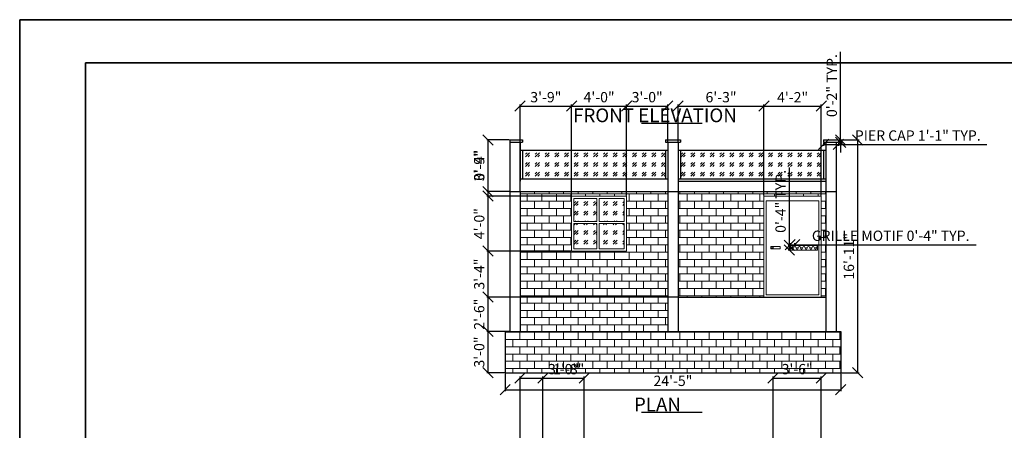
# Model space of a CAD drawing. Units: inches. Extents: x 1798 to 3594, y 1405 to 2404.
# Tile 5 of 6: x 1798 to 2658, y 2046 to 2404. Entities that reach past the tile are written whole.
import ezdxf

# ---------------------------------------------------------------- set-up
doc = ezdxf.new("R2010")
doc.units = ezdxf.units.IN
for name, color, linetype, lineweight in [('A-ANNO-DIMS', 6, 'Continuous', 18), ('A-ANNO-TITL', 6, 'Continuous', 25), ('A-ANNO-TTLB', 7, 'Continuous', 35), ('A-DOOR', 3, 'Continuous', 18), ('A-ELEV', 7, 'Continuous', 30), ('A-GLAZ', 4, 'Continuous', 18), ('A-GLAZ-PATT', 252, 'Continuous', 13), ('A-WALL-PATT', 252, 'Continuous', 13)]:
    doc.layers.add(name, color=color, linetype=linetype, lineweight=lineweight)
doc.styles.get("Standard").update_dxf_attribs({"font": 'arial.ttf'})
doc.dimstyles.new('ISO-25', dxfattribs={"dimtxt": 9, "dimasz": 9, "dimexe": 1.25, "dimexo": 0.625, "dimgap": 2, "dimtad": 1, "dimdec": 1, "dimlunit": 4, "dimtxsty": 'Standard', "dimblk": 'OBLIQUE', "dimcen": 2.5, "dimazin": 0, "dimtfac": 1, "dimtdec": 1, "dimtmove": 0, "dimatfit": 3, "dimfxl": 1, "dimarcsym": 0})
pattern_1 = [(45, (0, 1019.875), (8.485281, 0), [5, -7]), (45, (2.1213, 1019.875), (8.485281, 0), [2, -10]), (45, (0, 1021.996), (8.485281, 0), [2, -10])]

# ---------------------------------------------------------------- blocks, each defined once
blk = doc.blocks.new('PIER-CAP-13-ELEV')
for p, q in [((0, 2), (13, 2)), ((0, 2), (0, 0)), ((0, 0), (13, 0)), ((13, 2), (13, 0))]:
    blk.add_line(p, q)
blk = doc.blocks.new('DOOR-GRILLE-V-MOTIF')
for p, q in [((0, 4), (2, 0)), ((1, 2), (3, 2)), ((2, 0), (4, 4))]:
    blk.add_line(p, q)
blk = doc.blocks.new('_Oblique')
at = {"color": 0, "linetype": 'ByBlock', "lineweight": -2}
blk.add_line((-0.5, -0.5), (0.5, 0.5), dxfattribs=at)
blk = doc.blocks.new('*D15')
at = {"layer": 'A-ANNO-DIMS', "color": 0, "lineweight": -2, "transparency": 16777216}
for p, q in [((2471.14, 2207.46), (2471.14, 2208.69)), ((2471.14, 2207.44), (2475.14, 2207.44)), ((2475.14, 2207.46), (2475.14, 2208.69)), ((2475.14, 2207.44), (2633.67, 2207.44))]:
    blk.add_line(p, q, dxfattribs=at)
at = {"layer": 'Defpoints', "color": 0, "transparency": 16777216}
for p in [(2471.14, 2206.84), (2475.14, 2207.44), (2475.14, 2206.84)]:
    blk.add_point(p, dxfattribs=at)
at = {"layer": 'A-ANNO-DIMS', "color": 0, "lineweight": -2, "transparency": 16777216, "xscale": 9, "yscale": 9, "zscale": 9, "rotation": 180}
blk.add_blockref('_Oblique', (2471.14, 2207.44), dxfattribs=at)
at = {"layer": 'A-ANNO-DIMS', "color": 0, "lineweight": -2, "transparency": 16777216, "xscale": 9, "yscale": 9, "zscale": 9}
blk.add_blockref('_Oblique', (2475.14, 2207.44), dxfattribs=at)
at = {"layer": 'A-ANNO-DIMS', "color": 0, "transparency": 16777216, "insert": (2558.91, 2214.09), "char_height": 9, "attachment_point": 5}
blk.add_mtext('GRILLE MOTIF 0\'-4" TYP.', dxfattribs=at)
blk = doc.blocks.new('*D16')
at = {"layer": 'A-ANNO-DIMS', "color": 0, "lineweight": -2, "transparency": 16777216}
for p, q in [((2470.54, 2206.84), (2470.54, 2274.7)), ((2470.52, 2206.84), (2469.29, 2206.84)), ((2470.52, 2202.84), (2469.29, 2202.84)), ((2470.54, 2202.84), (2470.54, 2206.84))]:
    blk.add_line(p, q, dxfattribs=at)
at = {"layer": 'Defpoints', "color": 0, "transparency": 16777216}
for p in [(2470.54, 2206.84), (2471.14, 2206.84), (2471.14, 2202.84)]:
    blk.add_point(p, dxfattribs=at)
at = {"layer": 'A-ANNO-DIMS', "color": 0, "lineweight": -2, "transparency": 16777216, "xscale": 9, "yscale": 9, "zscale": 9}
for p, rotation in [((2470.54, 2206.84), 90), ((2470.54, 2202.84), 270)]:
    blk.add_blockref('_Oblique', p, dxfattribs=dict(at, rotation=rotation))
at = {"layer": 'A-ANNO-DIMS', "color": 0, "transparency": 16777216, "insert": (2463.95, 2245.27), "char_height": 9, "attachment_point": 5, "rotation": 90}
blk.add_mtext('0\'-4" TYP.', dxfattribs=at)
blk = doc.blocks.new('*D21')
at = {"layer": 'A-ANNO-DIMS', "color": 0, "lineweight": -2, "transparency": 16777216}
for p, q in [((2500.27, 2296.21), (2500.27, 2293.64)), ((2513.27, 2296.21), (2513.27, 2293.64)), ((2500.27, 2294.89), (2513.27, 2294.89)), ((2513.27, 2294.89), (2642.87, 2294.89))]:
    blk.add_line(p, q, dxfattribs=at)
at = {"layer": 'Defpoints', "color": 0, "transparency": 16777216}
for p in [(2500.27, 2296.84), (2513.27, 2296.84), (2513.27, 2294.89)]:
    blk.add_point(p, dxfattribs=at)
at = {"layer": 'A-ANNO-DIMS', "color": 0, "lineweight": -2, "transparency": 16777216, "xscale": 9, "yscale": 9, "zscale": 9, "rotation": 180}
blk.add_blockref('_Oblique', (2500.27, 2294.89), dxfattribs=at)
at = {"layer": 'A-ANNO-DIMS', "color": 0, "lineweight": -2, "transparency": 16777216, "xscale": 9, "yscale": 9, "zscale": 9}
blk.add_blockref('_Oblique', (2513.27, 2294.89), dxfattribs=at)
at = {"layer": 'A-ANNO-DIMS', "color": 0, "transparency": 16777216, "insert": (2582.57, 2301.54), "char_height": 9, "attachment_point": 5}
blk.add_mtext('PIER CAP 1\'-1" TYP.', dxfattribs=at)
blk = doc.blocks.new('*D22')
at = {"layer": 'A-ANNO-DIMS', "color": 0, "lineweight": -2, "transparency": 16777216}
for p, q in [((2515.22, 2298.84), (2515.22, 2375.7)), ((2513.9, 2298.84), (2516.47, 2298.84)), ((2513.9, 2296.84), (2516.47, 2296.84)), ((2515.22, 2296.84), (2515.22, 2298.84)), ((2515.22, 2296.84), (2515.22, 2287.84))]:
    blk.add_line(p, q, dxfattribs=at)
at = {"layer": 'Defpoints', "color": 0, "transparency": 16777216}
for p in [(2513.27, 2298.84), (2513.27, 2296.84), (2515.22, 2298.84)]:
    blk.add_point(p, dxfattribs=at)
at = {"layer": 'A-ANNO-DIMS', "color": 0, "lineweight": -2, "transparency": 16777216, "xscale": 9, "yscale": 9, "zscale": 9}
for p, rotation in [((2515.22, 2298.84), 270), ((2515.22, 2296.84), 90)]:
    blk.add_blockref('_Oblique', p, dxfattribs=dict(at, rotation=rotation))
at = {"layer": 'A-ANNO-DIMS', "color": 0, "transparency": 16777216, "insert": (2508.63, 2346.27), "char_height": 9, "attachment_point": 5, "rotation": 90}
blk.add_mtext('0\'-2" TYP.', dxfattribs=at)
blk = doc.blocks.new('*D42')
at = {"layer": 'A-ANNO-DIMS', "color": 0, "lineweight": -2, "transparency": 16777216}
for p, q in [((2235.27, 1867.44), (2235.27, 2092.43)), ((2235.27, 2091.18), (2255.27, 2091.18)), ((2255.27, 1867.44), (2255.27, 2092.43)), ((2255.27, 2091.18), (2291.35, 2091.18))]:
    blk.add_line(p, q, dxfattribs=at)
at = {"layer": 'Defpoints', "color": 0, "transparency": 16777216}
for p in [(2255.27, 2091.18), (2235.27, 1866.81), (2255.27, 1866.81)]:
    blk.add_point(p, dxfattribs=at)
at = {"layer": 'A-ANNO-DIMS', "color": 0, "lineweight": -2, "transparency": 16777216, "xscale": 9, "yscale": 9, "zscale": 9, "rotation": 180}
blk.add_blockref('_Oblique', (2235.27, 2091.18), dxfattribs=at)
at = {"layer": 'A-ANNO-DIMS', "color": 0, "lineweight": -2, "transparency": 16777216, "xscale": 9, "yscale": 9, "zscale": 9}
blk.add_blockref('_Oblique', (2255.27, 2091.18), dxfattribs=at)
at = {"layer": 'A-ANNO-DIMS', "color": 0, "transparency": 16777216, "insert": (2277.81, 2097.78), "char_height": 9, "attachment_point": 5}
blk.add_mtext('1\'-8"', dxfattribs=at)
blk = doc.blocks.new('*D43')
at = {"layer": 'A-ANNO-DIMS', "color": 0, "lineweight": -2, "transparency": 16777216}
for p, q in [((2255.27, 1867.44), (2255.27, 2092.43)), ((2255.27, 2091.18), (2291.27, 2091.18)), ((2291.27, 1867.44), (2291.27, 2092.43))]:
    blk.add_line(p, q, dxfattribs=at)
at = {"layer": 'Defpoints', "color": 0, "transparency": 16777216}
for p in [(2291.27, 2091.18), (2255.27, 1866.81), (2291.27, 1866.81)]:
    blk.add_point(p, dxfattribs=at)
at = {"layer": 'A-ANNO-DIMS', "color": 0, "lineweight": -2, "transparency": 16777216, "xscale": 9, "yscale": 9, "zscale": 9, "rotation": 180}
blk.add_blockref('_Oblique', (2255.27, 2091.18), dxfattribs=at)
at = {"layer": 'A-ANNO-DIMS', "color": 0, "lineweight": -2, "transparency": 16777216, "xscale": 9, "yscale": 9, "zscale": 9}
blk.add_blockref('_Oblique', (2291.27, 2091.18), dxfattribs=at)
at = {"layer": 'A-ANNO-DIMS', "color": 0, "transparency": 16777216, "insert": (2273.27, 2097.78), "char_height": 9, "attachment_point": 5}
blk.add_mtext('3\'-0"', dxfattribs=at)
blk = doc.blocks.new('*D47')
at = {"layer": 'A-ANNO-DIMS', "color": 0, "lineweight": -2, "transparency": 16777216}
for p, q in [((2456.27, 1666.44), (2456.27, 2092.43)), ((2456.27, 2091.18), (2498.27, 2091.18)), ((2498.27, 1666.44), (2498.27, 2092.43))]:
    blk.add_line(p, q, dxfattribs=at)
at = {"layer": 'Defpoints', "color": 0, "transparency": 16777216}
for p in [(2498.27, 2091.18), (2456.27, 1665.81), (2498.27, 1665.81)]:
    blk.add_point(p, dxfattribs=at)
at = {"layer": 'A-ANNO-DIMS', "color": 0, "lineweight": -2, "transparency": 16777216, "xscale": 9, "yscale": 9, "zscale": 9, "rotation": 180}
blk.add_blockref('_Oblique', (2456.27, 2091.18), dxfattribs=at)
at = {"layer": 'A-ANNO-DIMS', "color": 0, "lineweight": -2, "transparency": 16777216, "xscale": 9, "yscale": 9, "zscale": 9}
blk.add_blockref('_Oblique', (2498.27, 2091.18), dxfattribs=at)
at = {"layer": 'A-ANNO-DIMS', "color": 0, "transparency": 16777216, "insert": (2477.27, 2097.78), "char_height": 9, "attachment_point": 5}
blk.add_mtext('3\'-6"', dxfattribs=at)
blk = doc.blocks.new('*D53')
at = {"layer": 'A-ANNO-DIMS', "color": 0, "lineweight": -2, "transparency": 16777216}
for p, q in [((2222.27, 2095.21), (2222.27, 2079.69)), ((2515.27, 2095.21), (2515.27, 2079.69)), ((2222.27, 2080.94), (2515.27, 2080.94))]:
    blk.add_line(p, q, dxfattribs=at)
at = {"layer": 'Defpoints', "color": 0, "transparency": 16777216}
for p in [(2222.27, 2095.84), (2515.27, 2095.84), (2515.27, 2080.94)]:
    blk.add_point(p, dxfattribs=at)
at = {"layer": 'A-ANNO-DIMS', "color": 0, "lineweight": -2, "transparency": 16777216, "xscale": 9, "yscale": 9, "zscale": 9, "rotation": 180}
blk.add_blockref('_Oblique', (2222.27, 2080.94), dxfattribs=at)
at = {"layer": 'A-ANNO-DIMS', "color": 0, "lineweight": -2, "transparency": 16777216, "xscale": 9, "yscale": 9, "zscale": 9}
blk.add_blockref('_Oblique', (2515.27, 2080.94), dxfattribs=at)
at = {"layer": 'A-ANNO-DIMS', "color": 0, "transparency": 16777216, "insert": (2368.77, 2087.53), "char_height": 9, "attachment_point": 5}
blk.add_mtext('24\'-5"', dxfattribs=at)
blk = doc.blocks.new('*D54')
at = {"layer": 'A-ANNO-DIMS', "color": 0, "lineweight": -2, "transparency": 16777216}
for p, q in [((2513.9, 2298.84), (2531.42, 2298.84)), ((2530.17, 2095.84), (2530.17, 2298.84)), ((2515.9, 2095.84), (2531.42, 2095.84))]:
    blk.add_line(p, q, dxfattribs=at)
at = {"layer": 'Defpoints', "color": 0, "transparency": 16777216}
for p in [(2513.27, 2298.84), (2530.17, 2298.84), (2515.27, 2095.84)]:
    blk.add_point(p, dxfattribs=at)
at = {"layer": 'A-ANNO-DIMS', "color": 0, "lineweight": -2, "transparency": 16777216, "xscale": 9, "yscale": 9, "zscale": 9}
for p, rotation in [((2530.17, 2298.84), 90), ((2530.17, 2095.84), 270)]:
    blk.add_blockref('_Oblique', p, dxfattribs=dict(at, rotation=rotation))
at = {"layer": 'A-ANNO-DIMS', "color": 0, "transparency": 16777216, "insert": (2523.58, 2197.34), "char_height": 9, "attachment_point": 5, "rotation": 90}
blk.add_mtext('16\'-11"', dxfattribs=at)
blk = doc.blocks.new('*D55')
at = {"layer": 'A-ANNO-DIMS', "color": 0, "lineweight": -2, "transparency": 16777216}
for p, q in [((2221.65, 2131.84), (2206.12, 2131.84)), ((2207.37, 2095.84), (2207.37, 2131.84)), ((2221.65, 2095.84), (2206.12, 2095.84))]:
    blk.add_line(p, q, dxfattribs=at)
at = {"layer": 'Defpoints', "color": 0, "transparency": 16777216}
for p in [(2207.37, 2131.84), (2222.27, 2131.84), (2222.27, 2095.84)]:
    blk.add_point(p, dxfattribs=at)
at = {"layer": 'A-ANNO-DIMS', "color": 0, "lineweight": -2, "transparency": 16777216, "xscale": 9, "yscale": 9, "zscale": 9}
for p, rotation in [((2207.37, 2131.84), 90), ((2207.37, 2095.84), 270)]:
    blk.add_blockref('_Oblique', p, dxfattribs=dict(at, rotation=rotation))
at = {"layer": 'A-ANNO-DIMS', "color": 0, "transparency": 16777216, "insert": (2200.77, 2113.84), "char_height": 9, "attachment_point": 5, "rotation": 90}
blk.add_mtext('3\'-0"', dxfattribs=at)
blk = doc.blocks.new('*D56')
at = {"layer": 'A-ANNO-DIMS', "color": 0, "lineweight": -2, "transparency": 16777216}
for p, q in [((2372.65, 2161.84), (2206.12, 2161.84)), ((2207.37, 2131.84), (2207.37, 2161.84)), ((2225.65, 2131.84), (2206.12, 2131.84))]:
    blk.add_line(p, q, dxfattribs=at)
at = {"layer": 'Defpoints', "color": 0, "transparency": 16777216}
for p in [(2207.37, 2161.84), (2373.27, 2161.84), (2226.27, 2131.84)]:
    blk.add_point(p, dxfattribs=at)
at = {"layer": 'A-ANNO-DIMS', "color": 0, "lineweight": -2, "transparency": 16777216, "xscale": 9, "yscale": 9, "zscale": 9}
for p, rotation in [((2207.37, 2161.84), 90), ((2207.37, 2131.84), 270)]:
    blk.add_blockref('_Oblique', p, dxfattribs=dict(at, rotation=rotation))
at = {"layer": 'A-ANNO-DIMS', "color": 0, "transparency": 16777216, "insert": (2200.78, 2146.84), "char_height": 9, "attachment_point": 5, "rotation": 90}
blk.add_mtext('2\'-6"', dxfattribs=at)
blk = doc.blocks.new('*D57')
at = {"layer": 'A-ANNO-DIMS', "color": 0, "lineweight": -2, "transparency": 16777216}
for p, q in [((2279.65, 2201.84), (2206.12, 2201.84)), ((2207.37, 2161.84), (2207.37, 2201.84)), ((2372.65, 2161.84), (2206.12, 2161.84))]:
    blk.add_line(p, q, dxfattribs=at)
at = {"layer": 'Defpoints', "color": 0, "transparency": 16777216}
for p in [(2207.37, 2201.84), (2280.27, 2201.84), (2373.27, 2161.84)]:
    blk.add_point(p, dxfattribs=at)
at = {"layer": 'A-ANNO-DIMS', "color": 0, "lineweight": -2, "transparency": 16777216, "xscale": 9, "yscale": 9, "zscale": 9}
for p, rotation in [((2207.37, 2201.84), 90), ((2207.37, 2161.84), 270)]:
    blk.add_blockref('_Oblique', p, dxfattribs=dict(at, rotation=rotation))
at = {"layer": 'A-ANNO-DIMS', "color": 0, "transparency": 16777216, "insert": (2200.77, 2181.84), "char_height": 9, "attachment_point": 5, "rotation": 90}
blk.add_mtext('3\'-4"', dxfattribs=at)
blk = doc.blocks.new('*D58')
at = {"layer": 'A-ANNO-DIMS', "color": 0, "lineweight": -2, "transparency": 16777216}
for p, q in [((2279.65, 2249.84), (2206.12, 2249.84)), ((2207.37, 2201.84), (2207.37, 2249.84)), ((2279.65, 2201.84), (2206.12, 2201.84))]:
    blk.add_line(p, q, dxfattribs=at)
at = {"layer": 'Defpoints', "color": 0, "transparency": 16777216}
for p in [(2207.37, 2249.84), (2280.27, 2249.84), (2280.27, 2201.84)]:
    blk.add_point(p, dxfattribs=at)
at = {"layer": 'A-ANNO-DIMS', "color": 0, "lineweight": -2, "transparency": 16777216, "xscale": 9, "yscale": 9, "zscale": 9}
for p, rotation in [((2207.37, 2249.84), 90), ((2207.37, 2201.84), 270)]:
    blk.add_blockref('_Oblique', p, dxfattribs=dict(at, rotation=rotation))
at = {"layer": 'A-ANNO-DIMS', "color": 0, "transparency": 16777216, "insert": (2200.78, 2225.84), "char_height": 9, "attachment_point": 5, "rotation": 90}
blk.add_mtext('4\'-0"', dxfattribs=at)
blk = doc.blocks.new('*D59')
at = {"layer": 'A-ANNO-DIMS', "color": 0, "lineweight": -2, "transparency": 16777216}
for p, q in [((2207.37, 2253.84), (2207.37, 2290.76)), ((2225.65, 2253.84), (2206.12, 2253.84)), ((2207.37, 2249.84), (2207.37, 2253.84)), ((2279.65, 2249.84), (2206.12, 2249.84))]:
    blk.add_line(p, q, dxfattribs=at)
at = {"layer": 'Defpoints', "color": 0, "transparency": 16777216}
for p in [(2207.37, 2253.84), (2226.27, 2253.84), (2280.27, 2249.84)]:
    blk.add_point(p, dxfattribs=at)
at = {"layer": 'A-ANNO-DIMS', "color": 0, "lineweight": -2, "transparency": 16777216, "xscale": 9, "yscale": 9, "zscale": 9}
for p, rotation in [((2207.37, 2253.84), 90), ((2207.37, 2249.84), 270)]:
    blk.add_blockref('_Oblique', p, dxfattribs=dict(at, rotation=rotation))
at = {"layer": 'A-ANNO-DIMS', "color": 0, "transparency": 16777216, "insert": (2200.78, 2276.8), "char_height": 9, "attachment_point": 5, "rotation": 90}
blk.add_mtext('0\'-4"', dxfattribs=at)
blk = doc.blocks.new('*D60')
at = {"layer": 'A-ANNO-DIMS', "color": 0, "lineweight": -2, "transparency": 16777216}
for p, q in [((2225.65, 2298.84), (2206.12, 2298.84)), ((2207.37, 2253.84), (2207.37, 2298.84)), ((2225.65, 2253.84), (2206.12, 2253.84))]:
    blk.add_line(p, q, dxfattribs=at)
at = {"layer": 'Defpoints', "color": 0, "transparency": 16777216}
for p in [(2207.37, 2298.84), (2226.27, 2298.84), (2226.27, 2253.84)]:
    blk.add_point(p, dxfattribs=at)
at = {"layer": 'A-ANNO-DIMS', "color": 0, "lineweight": -2, "transparency": 16777216, "xscale": 9, "yscale": 9, "zscale": 9}
for p, rotation in [((2207.37, 2298.84), 90), ((2207.37, 2253.84), 270)]:
    blk.add_blockref('_Oblique', p, dxfattribs=dict(at, rotation=rotation))
at = {"layer": 'A-ANNO-DIMS', "color": 0, "transparency": 16777216, "insert": (2200.77, 2276.34), "char_height": 9, "attachment_point": 5, "rotation": 90}
blk.add_mtext('3\'-9"', dxfattribs=at)
blk = doc.blocks.new('*D61')
at = {"layer": 'A-ANNO-DIMS', "color": 0, "lineweight": -2, "transparency": 16777216}
for p, q in [((2235.27, 2254.46), (2235.27, 2329.66)), ((2235.27, 2328.41), (2280.27, 2328.41)), ((2280.27, 2250.46), (2280.27, 2329.66))]:
    blk.add_line(p, q, dxfattribs=at)
at = {"layer": 'Defpoints', "color": 0, "transparency": 16777216}
for p in [(2280.27, 2328.41), (2235.27, 2253.84), (2280.27, 2249.84)]:
    blk.add_point(p, dxfattribs=at)
at = {"layer": 'A-ANNO-DIMS', "color": 0, "lineweight": -2, "transparency": 16777216, "xscale": 9, "yscale": 9, "zscale": 9, "rotation": 180}
blk.add_blockref('_Oblique', (2235.27, 2328.41), dxfattribs=at)
at = {"layer": 'A-ANNO-DIMS', "color": 0, "lineweight": -2, "transparency": 16777216, "xscale": 9, "yscale": 9, "zscale": 9}
blk.add_blockref('_Oblique', (2280.27, 2328.41), dxfattribs=at)
at = {"layer": 'A-ANNO-DIMS', "color": 0, "transparency": 16777216, "insert": (2257.77, 2335.01), "char_height": 9, "attachment_point": 5}
blk.add_mtext('3\'-9"', dxfattribs=at)
blk = doc.blocks.new('*D62')
at = {"layer": 'A-ANNO-DIMS', "color": 0, "lineweight": -2, "transparency": 16777216}
for p, q in [((2280.27, 2250.46), (2280.27, 2329.66)), ((2280.27, 2328.41), (2328.27, 2328.41)), ((2328.27, 2250.46), (2328.27, 2329.66))]:
    blk.add_line(p, q, dxfattribs=at)
at = {"layer": 'Defpoints', "color": 0, "transparency": 16777216}
for p in [(2328.27, 2328.41), (2280.27, 2249.84), (2328.27, 2249.84)]:
    blk.add_point(p, dxfattribs=at)
at = {"layer": 'A-ANNO-DIMS', "color": 0, "lineweight": -2, "transparency": 16777216, "xscale": 9, "yscale": 9, "zscale": 9, "rotation": 180}
blk.add_blockref('_Oblique', (2280.27, 2328.41), dxfattribs=at)
at = {"layer": 'A-ANNO-DIMS', "color": 0, "lineweight": -2, "transparency": 16777216, "xscale": 9, "yscale": 9, "zscale": 9}
blk.add_blockref('_Oblique', (2328.27, 2328.41), dxfattribs=at)
at = {"layer": 'A-ANNO-DIMS', "color": 0, "transparency": 16777216, "insert": (2304.27, 2335.01), "char_height": 9, "attachment_point": 5}
blk.add_mtext('4\'-0"', dxfattribs=at)
blk = doc.blocks.new('*D63')
at = {"layer": 'A-ANNO-DIMS', "color": 0, "lineweight": -2, "transparency": 16777216}
for p, q in [((2328.27, 2250.46), (2328.27, 2329.66)), ((2328.27, 2328.41), (2364.27, 2328.41)), ((2364.27, 2297.46), (2364.27, 2329.66))]:
    blk.add_line(p, q, dxfattribs=at)
at = {"layer": 'Defpoints', "color": 0, "transparency": 16777216}
for p in [(2364.27, 2328.41), (2364.27, 2296.84), (2328.27, 2249.84)]:
    blk.add_point(p, dxfattribs=at)
at = {"layer": 'A-ANNO-DIMS', "color": 0, "lineweight": -2, "transparency": 16777216, "xscale": 9, "yscale": 9, "zscale": 9, "rotation": 180}
blk.add_blockref('_Oblique', (2328.27, 2328.41), dxfattribs=at)
at = {"layer": 'A-ANNO-DIMS', "color": 0, "lineweight": -2, "transparency": 16777216, "xscale": 9, "yscale": 9, "zscale": 9}
blk.add_blockref('_Oblique', (2364.27, 2328.41), dxfattribs=at)
at = {"layer": 'A-ANNO-DIMS', "color": 0, "transparency": 16777216, "insert": (2346.27, 2335.01), "char_height": 9, "attachment_point": 5}
blk.add_mtext('3\'-0"', dxfattribs=at)
blk = doc.blocks.new('*D64')
at = {"layer": 'A-ANNO-DIMS', "color": 0, "lineweight": -2, "transparency": 16777216}
for p, q in [((2373.27, 2297.46), (2373.27, 2329.66)), ((2373.27, 2328.41), (2448.27, 2328.41)), ((2448.27, 2250.46), (2448.27, 2329.66))]:
    blk.add_line(p, q, dxfattribs=at)
at = {"layer": 'Defpoints', "color": 0, "transparency": 16777216}
for p in [(2448.27, 2328.41), (2373.27, 2296.84), (2448.27, 2249.84)]:
    blk.add_point(p, dxfattribs=at)
at = {"layer": 'A-ANNO-DIMS', "color": 0, "lineweight": -2, "transparency": 16777216, "xscale": 9, "yscale": 9, "zscale": 9, "rotation": 180}
blk.add_blockref('_Oblique', (2373.27, 2328.41), dxfattribs=at)
at = {"layer": 'A-ANNO-DIMS', "color": 0, "lineweight": -2, "transparency": 16777216, "xscale": 9, "yscale": 9, "zscale": 9}
blk.add_blockref('_Oblique', (2448.27, 2328.41), dxfattribs=at)
at = {"layer": 'A-ANNO-DIMS', "color": 0, "transparency": 16777216, "insert": (2410.77, 2335.01), "char_height": 9, "attachment_point": 5}
blk.add_mtext('6\'-3"', dxfattribs=at)
blk = doc.blocks.new('*D65')
at = {"layer": 'A-ANNO-DIMS', "color": 0, "lineweight": -2, "transparency": 16777216}
for p, q in [((2448.27, 2250.46), (2448.27, 2329.66)), ((2448.27, 2328.41), (2498.27, 2328.41)), ((2498.27, 2250.46), (2498.27, 2329.66))]:
    blk.add_line(p, q, dxfattribs=at)
at = {"layer": 'Defpoints', "color": 0, "transparency": 16777216}
for p in [(2498.27, 2328.41), (2448.27, 2249.84), (2498.27, 2249.84)]:
    blk.add_point(p, dxfattribs=at)
at = {"layer": 'A-ANNO-DIMS', "color": 0, "lineweight": -2, "transparency": 16777216, "xscale": 9, "yscale": 9, "zscale": 9, "rotation": 180}
blk.add_blockref('_Oblique', (2448.27, 2328.41), dxfattribs=at)
at = {"layer": 'A-ANNO-DIMS', "color": 0, "lineweight": -2, "transparency": 16777216, "xscale": 9, "yscale": 9, "zscale": 9}
blk.add_blockref('_Oblique', (2498.27, 2328.41), dxfattribs=at)
at = {"layer": 'A-ANNO-DIMS', "color": 0, "transparency": 16777216, "insert": (2473.27, 2334.93), "char_height": 9, "attachment_point": 5}
blk.add_mtext('4\'-2"', dxfattribs=at)

msp = doc.modelspace()

# ---------------------------------------------------------------- hatches: boundary and pattern name
at = {"layer": 'A-GLAZ-PATT'}
h = msp.add_hatch(dxfattribs=at)
h.set_pattern_fill('GOST_GLASS', color=256)
h.set_pattern_definition(pattern_1)
h.paths.add_polyline_path([(2237.27, 2289.84), (2237.27, 2264.84), (2362.27, 2264.84), (2362.27, 2289.84)])
h.paths.add_polyline_path([(2375.27, 2289.84), (2375.27, 2264.84), (2500.27, 2264.84), (2500.27, 2289.84)])
h = msp.add_hatch(dxfattribs=at)
h.set_pattern_fill('GOST_GLASS', color=256)
h.set_pattern_definition(pattern_1)
h.paths.add_polyline_path([(2282.27, 2247.84), (2282.27, 2227.84), (2302.27, 2227.84), (2302.27, 2247.84)])
h.paths.add_polyline_path([(2304.27, 2227.84), (2326.27, 2227.84), (2326.27, 2247.84), (2304.27, 2247.84)])
h.paths.add_polyline_path([(2304.27, 2225.84), (2304.27, 2203.84), (2326.27, 2203.84), (2326.27, 2225.84)])
h.paths.add_polyline_path([(2282.27, 2203.84), (2302.27, 2203.84), (2302.27, 2225.84), (2282.27, 2225.84)])
at = {"layer": 'A-WALL-PATT'}
h = msp.add_hatch(dxfattribs=at)
h.set_pattern_fill('BRICK', color=256)
h.set_pattern_definition([(0, (0, 1019.875), (0, 6.35), []), (90, (0, 1019.875), (-12.7, 8e-16), [6.35, -6.35]), (90, (6.35, 1019.875), (-12.7, 8e-16), [-6.35, 6.35])])
h.paths.add_polyline_path([(2515.27, 2131.84), (2222.27, 2131.84), (2222.27, 2095.84), (2515.27, 2095.84)])
h.paths.add_polyline_path([(2364.27, 2253.84), (2235.27, 2253.84), (2235.27, 2131.84), (2364.27, 2131.84)])
h.paths.add_polyline_path([(2280.27, 2201.84), (2280.27, 2249.84), (2328.27, 2249.84), (2328.27, 2201.84)], flags=16)
h.paths.add_polyline_path([(2282.27, 2203.84), (2282.27, 2225.84), (2302.27, 2225.84), (2302.27, 2203.84)], flags=0)
h.paths.add_polyline_path([(2304.27, 2203.84), (2304.27, 2225.84), (2326.27, 2225.84), (2326.27, 2203.84)], flags=0)
h.paths.add_polyline_path([(2282.27, 2227.84), (2282.27, 2247.84), (2302.27, 2247.84), (2302.27, 2227.84)], flags=0)
h.paths.add_polyline_path([(2304.27, 2227.84), (2304.27, 2247.84), (2326.27, 2247.84), (2326.27, 2227.84)], flags=0)
h.paths.add_polyline_path([(2448.27, 2249.84), (2496.27, 2249.84), (2498.27, 2249.84), (2498.27, 2161.84), (2502.27, 2161.84), (2502.27, 2253.84), (2373.27, 2253.84), (2373.27, 2161.84), (2448.27, 2161.84)])

# ---------------------------------------------------------------- linework, layer by layer
at = {"layer": 'A-ANNO-TITL'}
for p, q in [((2341.44, 2313.51), (2394.35, 2313.51)), ((2341.44, 2061.28), (2394.35, 2061.28))]:
    msp.add_line(p, q, dxfattribs=at)
at = {"layer": 'A-ANNO-TTLB'}
for points in [[(1798.35, 2403.73), (3594.23, 2403.73), (3594.23, 1405.28), (1798.35, 1405.28)], [(1855.68, 2366.05), (3540.6, 2366.05), (3540.6, 1444.98), (1855.68, 1444.98)]]:
    msp.add_lwpolyline(points, close=True, dxfattribs=at)
at = {"layer": 'A-DOOR'}
for p, q in [((2448.27, 2249.84), (2448.27, 2161.84)), ((2448.27, 2249.84), (2498.27, 2249.84)), ((2448.27, 2249.84), (2496.27, 2249.84)), ((2450.27, 2245.84), (2450.27, 2163.84)), ((2450.27, 2245.84), (2496.27, 2245.84)), ((2496.27, 2245.84), (2496.27, 2163.84)), ((2498.27, 2249.84), (2498.27, 2161.84)), ((2454.27, 2205.84), (2454.27, 2203.84)), ((2454.27, 2205.84), (2462.27, 2205.84)), ((2454.27, 2204.84), (2456.27, 2204.84)), ((2454.27, 2203.84), (2462.27, 2203.84)), ((2456.27, 2205.84), (2456.27, 2203.84)), ((2456.27, 2205.84), (2456.27, 2203.84)), ((2462.27, 2205.84), (2462.27, 2203.84)), ((2471.14, 2206.84), (2471.14, 2202.84)), ((2471.14, 2206.84), (2495.14, 2206.84)), ((2471.14, 2202.84), (2495.14, 2202.84)), ((2495.14, 2206.84), (2495.14, 2202.84)), ((2450.27, 2163.84), (2496.27, 2163.84))]:
    msp.add_line(p, q, dxfattribs=at)
at = {"layer": 'A-ELEV'}
for p, q in [((2226.27, 2298.84), (2237.27, 2298.84)), ((2226.27, 2298.84), (2226.27, 2131.84)), ((2226.27, 2296.84), (2237.27, 2296.84)), ((2235.27, 2296.84), (2235.27, 2262.84)), ((2237.27, 2298.84), (2237.27, 2296.84)), ((2364.27, 2296.84), (2364.27, 2262.84)), ((2373.27, 2296.84), (2373.27, 2262.84)), ((2502.27, 2296.84), (2502.27, 2262.84)), ((2511.27, 2296.84), (2511.27, 2131.84)), ((2235.27, 2289.84), (2364.27, 2289.84)), ((2237.27, 2289.84), (2237.27, 2264.84)), ((2362.27, 2289.84), (2362.27, 2264.84)), ((2373.27, 2289.84), (2502.27, 2289.84)), ((2375.27, 2289.84), (2375.27, 2264.84)), ((2500.27, 2289.84), (2500.27, 2264.84)), ((2235.27, 2264.84), (2364.27, 2264.84)), ((2364.27, 2262.84), (2364.27, 2131.84)), ((2373.27, 2264.84), (2502.27, 2264.84)), ((2373.27, 2262.84), (2373.27, 2131.84)), ((2373.27, 2262.84), (2502.27, 2262.84)), ((2502.27, 2262.84), (2502.27, 2131.84)), ((2226.27, 2253.84), (2502.27, 2253.84)), ((2235.27, 2253.84), (2235.27, 2131.84)), ((2502.27, 2253.84), (2511.27, 2253.84)), ((2373.27, 2161.84), (2502.27, 2161.84)), ((2222.27, 2131.84), (2515.27, 2131.84)), ((2222.27, 2131.84), (2222.27, 2095.84)), ((2515.27, 2131.84), (2515.27, 2095.84)), ((2222.27, 2095.84), (2515.27, 2095.84))]:
    msp.add_line(p, q, dxfattribs=at)
at = {"layer": 'A-GLAZ'}
for p, q in [((2280.27, 2249.84), (2280.27, 2201.84)), ((2280.27, 2249.84), (2328.27, 2249.84)), ((2282.27, 2247.84), (2302.27, 2247.84)), ((2282.27, 2247.84), (2282.27, 2227.84)), ((2302.27, 2247.84), (2302.27, 2227.84)), ((2304.27, 2247.84), (2304.27, 2227.84)), ((2304.27, 2247.84), (2326.27, 2247.84)), ((2326.27, 2247.84), (2326.27, 2227.84)), ((2328.27, 2249.84), (2328.27, 2201.84)), ((2282.27, 2227.84), (2302.27, 2227.84)), ((2304.27, 2227.84), (2326.27, 2227.84)), ((2282.27, 2225.84), (2302.27, 2225.84)), ((2282.27, 2225.84), (2282.27, 2203.84)), ((2302.27, 2225.84), (2302.27, 2203.84)), ((2304.27, 2225.84), (2326.27, 2225.84)), ((2304.27, 2225.84), (2304.27, 2203.84)), ((2326.27, 2225.84), (2326.27, 2203.84)), ((2280.27, 2201.84), (2328.27, 2201.84)), ((2282.27, 2203.84), (2302.27, 2203.84)), ((2304.27, 2203.84), (2326.27, 2203.84))]:
    msp.add_line(p, q, dxfattribs=at)

# ---------------------------------------------------------------- block references
at = {"layer": 'A-DOOR'}
for p in [(2471.14, 2202.84), (2475.14, 2202.84), (2479.14, 2202.84), (2483.14, 2202.84), (2487.14, 2202.84), (2491.14, 2202.84)]:
    msp.add_blockref('DOOR-GRILLE-V-MOTIF', p, dxfattribs=at)
at = {"layer": 'A-ELEV'}
for p in [(2362.27, 2296.84), (2500.27, 2296.84)]:
    msp.add_blockref('PIER-CAP-13-ELEV', p, dxfattribs=at)

# ---------------------------------------------------------------- texts
at = {"layer": 'A-ANNO-TITL'}
for s, p in [('            FRONT ELEVATION', (2237.55, 2314.34)), ('            PLAN', (2290.72, 2062.11))]:
    msp.add_text(s, height=12, dxfattribs=at).set_placement(p)

# ---------------------------------------------------------------- dimensions: what is measured, and where the dimension line sits
at = {"layer": 'A-ANNO-DIMS'}
for base, p1, p2, picture, middle in [((2515.22, 2298.84), (2513.27, 2296.84), (2513.27, 2298.84), '*D22', (2508.63, 2346.27)), ((2470.54, 2206.84), (2471.14, 2202.84), (2471.14, 2206.84), '*D16', (2463.95, 2245.27))]:
    dim = msp.add_linear_dim(base=base, p1=p1, p2=p2, angle=90, text='<> TYP.', dimstyle='ISO-25', override={"dimdec": 1, "dimlfac": 1, "dimrnd": 0, "dimzin": 1, "dimdsep": 46, "dimlunit": 4, "dimfrac": 2}, dxfattribs=at)
    dim.commit()
    dim.dimension.update_dxf_attribs({"geometry": picture, "text_midpoint": middle})
for base, p1, p2, picture, middle in [((2280.27, 2328.41), (2235.27, 2253.84), (2280.27, 2249.84), '*D61', (2257.77, 2335.01)), ((2328.27, 2328.41), (2280.27, 2249.84), (2328.27, 2249.84), '*D62', (2304.27, 2335.01)), ((2364.27, 2328.41), (2328.27, 2249.84), (2364.27, 2296.84), '*D63', (2346.27, 2335.01)), ((2448.27, 2328.41), (2373.27, 2296.84), (2448.27, 2249.84), '*D64', (2410.77, 2335.01)), ((2498.27, 2328.41), (2448.27, 2249.84), (2498.27, 2249.84), '*D65', (2473.27, 2334.93)), ((2255.27, 2091.18), (2235.27, 1866.81), (2255.27, 1866.81), '*D42', (2277.81, 2097.78)), ((2291.27, 2091.18), (2255.27, 1866.81), (2291.27, 1866.81), '*D43', (2273.27, 2097.78)), ((2498.27, 2091.18), (2456.27, 1665.81), (2498.27, 1665.81), '*D47', (2477.27, 2097.78)), ((2515.27, 2080.94), (2222.27, 2095.84), (2515.27, 2095.84), '*D53', (2368.77, 2087.53))]:
    dim = msp.add_linear_dim(base=base, p1=p1, p2=p2, dimstyle='ISO-25', override={"dimdec": 1, "dimlfac": 1, "dimrnd": 0, "dimzin": 1, "dimdsep": 46, "dimlunit": 4, "dimfrac": 2}, dxfattribs=at)
    dim.commit()
    dim.dimension.update_dxf_attribs({"geometry": picture, "text_midpoint": middle})
for base, p1, p2, text, picture, middle in [((2513.27, 2294.89), (2500.27, 2296.84), (2513.27, 2296.84), 'PIER CAP <> TYP.', '*D21', (2582.57, 2301.54)), ((2475.14, 2207.44), (2471.14, 2206.84), (2475.14, 2206.84), 'GRILLE MOTIF <> TYP.', '*D15', (2558.91, 2214.09))]:
    dim = msp.add_linear_dim(base=base, p1=p1, p2=p2, text=text, dimstyle='ISO-25', override={"dimdec": 1, "dimlfac": 1, "dimrnd": 0, "dimzin": 1, "dimdsep": 46, "dimlunit": 4, "dimfrac": 2}, dxfattribs=at)
    dim.commit()
    dim.dimension.update_dxf_attribs({"geometry": picture, "text_midpoint": middle})
for base, p1, p2, picture, middle in [((2207.37, 2298.84), (2226.27, 2253.84), (2226.27, 2298.84), '*D60', (2200.77, 2276.34)), ((2530.17, 2298.84), (2515.27, 2095.84), (2513.27, 2298.84), '*D54', (2523.58, 2197.34)), ((2207.37, 2253.84), (2280.27, 2249.84), (2226.27, 2253.84), '*D59', (2200.78, 2276.8)), ((2207.37, 2249.84), (2280.27, 2201.84), (2280.27, 2249.84), '*D58', (2200.78, 2225.84)), ((2207.37, 2201.84), (2373.27, 2161.84), (2280.27, 2201.84), '*D57', (2200.77, 2181.84)), ((2207.37, 2161.84), (2226.27, 2131.84), (2373.27, 2161.84), '*D56', (2200.78, 2146.84)), ((2207.37, 2131.84), (2222.27, 2095.84), (2222.27, 2131.84), '*D55', (2200.77, 2113.84))]:
    dim = msp.add_linear_dim(base=base, p1=p1, p2=p2, angle=90, dimstyle='ISO-25', override={"dimdec": 1, "dimlfac": 1, "dimrnd": 0, "dimzin": 1, "dimdsep": 46, "dimlunit": 4, "dimfrac": 2}, dxfattribs=at)
    dim.commit()
    dim.dimension.update_dxf_attribs({"geometry": picture, "text_midpoint": middle})

doc.saveas('drawing.dxf')
